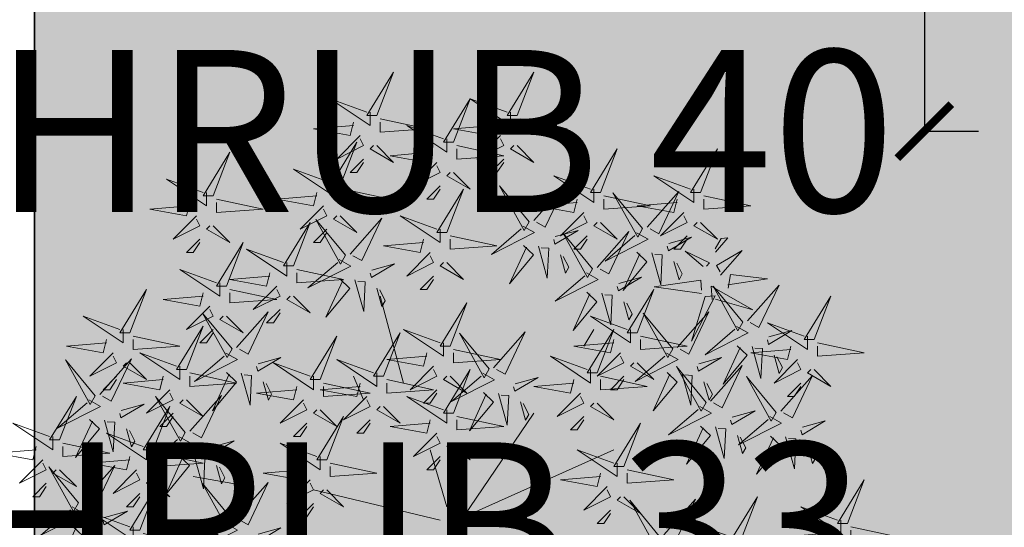
# Model space of a CAD drawing. Units: inches. Extents: x 1704 to 6393, y -157 to 1172.
# Tile 13 of 122: x 1898 to 1934, y 138 to 157. Entities that reach past the tile are written whole.
import ezdxf

# ---------------------------------------------------------------- set-up
doc = ezdxf.new("R2010")
doc.units = ezdxf.units.IN
doc.header["$MEASUREMENT"] = 0
for name, color, linetype, lineweight in [('A-ANNO-DIMS', 7, 'Continuous', 13), ('C-PROP', 7, 'Continuous', 35), ('L-shrub', 74, 'Continuous', 18)]:
    doc.layers.add(name, color=color, linetype=linetype, lineweight=lineweight)
doc.layers.add('L-PLNT-PATT', color=253, linetype='Continuous', lineweight=13, true_color=0x9abc8f)
doc.styles.get("Standard").update_dxf_attribs({"font": 'arial.ttf'})
doc.dimstyles.get("Standard").update_dxf_attribs({"dimtxt": 6, "dimasz": 2, "dimexe": 0.18, "dimexo": 0.0625, "dimgap": 0.09, "dimtad": 0, "dimtih": 1, "dimtoh": 1, "dimdec": 1, "dimzin": 0, "dimdsep": 46, "dimlunit": 3, "dimtxsty": 'Standard', "dimblk": 'ARCHTICK', "dimcen": 0.09, "dimadec": 0, "dimazin": 0, "dimtfac": 1, "dimtdec": 1, "dimtofl": 0, "dimtmove": 0, "dimatfit": 3, "dimfxl": 1, "dimtolj": 1, "dimtzin": 0, "dimarcsym": 0})

# ---------------------------------------------------------------- blocks, each defined once
blk = doc.blocks.new('autumn shrub')
at = {"layer": 'L-shrub'}
for p, q in [((11.54, 1.92), (51.94, 98)), ((1.92, -3.84), (-38.48, 86.47)), ((-98.12, 69.17), (-107.74, 74.94)), ((0, 0), (-59.64, 40.35)), ((71.18, 17.29), (98.12, 26.9)), ((9.62, -3.84), (71.18, 17.29)), ((11.54, -5.76), (55.79, 0)), ((-5.77, -9.61), (-38.48, -19.21)), ((1.92, -13.45), (-15.39, -86.47)), ((17.31, -26.9), (25.01, -40.35)), ((-76.95, -34.59), (-126.97, -48.04)), ((-67.33, -57.64), (-80.8, -63.41)), ((46.17, -69.17), (63.49, -101.84)), ((-17.31, -122.97), (-23.09, -155.64))]:
    blk.add_line(p, q, dxfattribs=at)
for points in [[(5.77, 222.89), (11.54, 249.79), (13.47, 222.89), (7.7, 222.89)], [(-100.04, 203.68), (-94.27, 230.58), (-92.34, 203.68), (-98.12, 203.68)], [(3.85, 220.97), (-21.16, 230.58), (3.85, 215.21), (3.85, 220.97)], [(21.16, 220.97), (30.78, 230.58), (23.09, 217.13), (21.16, 219.05)], [(1.92, 217.13), (9.62, 217.13), (-5.77, 194.07), (1.92, 215.21)], [(98.12, 194.07), (103.89, 220.97), (105.81, 194.07), (100.04, 194.07)], [(-101.96, 201.75), (-126.97, 211.36), (-101.96, 195.99), (-101.96, 201.75)], [(-84.65, 201.75), (-75.03, 211.36), (-82.73, 197.91), (-84.65, 199.83)], [(15.39, 211.36), (28.86, 197.91), (21.16, 213.28), (17.31, 211.36)], [(28.86, 213.28), (36.55, 205.6), (36.55, 209.44), (30.78, 213.28)], [(-51.51, 194.97), (-55.15, 208.07), (-47.22, 194.76), (-49.84, 194.03)], [(7.7, 207.52), (15.39, 205.6), (11.54, 184.46), (9.62, 207.52)], [(46.17, 180.62), (51.94, 207.52), (53.87, 180.62), (48.1, 180.62)], [(-60.75, 182.51), (-81.34, 200.76), (-56.96, 189.22), (-59.8, 184.19)], [(-41.04, 197.9), (-30.56, 200.83), (-33.91, 202.71), (-40.09, 199.58)], [(96.19, 192.15), (71.18, 201.75), (96.19, 186.38), (96.19, 192.15)], [(113.51, 192.15), (123.13, 201.75), (115.43, 188.3), (113.51, 190.23)], [(-103.89, 197.91), (-96.19, 197.91), (-111.58, 174.85), (-103.89, 195.99)], [(-90.42, 192.15), (-76.95, 178.7), (-84.65, 194.07), (-88.5, 192.15)], [(-76.95, 194.07), (-69.26, 186.38), (-69.26, 190.23), (-75.03, 194.07)], [(-103.45, 175.76), (-107.1, 188.86), (-99.16, 175.55), (-101.78, 174.81)], [(-98.12, 188.3), (-90.42, 186.38), (-94.27, 165.25), (-96.19, 188.3)], [(-45.98, 185.23), (-27.65, 190.35), (-44.82, 191.2), (-45.03, 186.9)], [(15.39, 161.4), (21.16, 188.3), (23.09, 161.4), (17.31, 161.4)], [(44.25, 178.7), (19.24, 188.3), (44.25, 172.93), (44.25, 178.7)], [(61.56, 178.7), (71.18, 188.3), (63.49, 174.85), (61.56, 176.78)], [(94.27, 188.3), (101.96, 188.3), (86.57, 165.25), (94.27, 186.38)], [(-112.69, 163.3), (-133.28, 181.54), (-108.91, 170), (-111.74, 164.97)], [(-92.98, 178.69), (-82.5, 181.61), (-85.85, 183.5), (-92.03, 180.36)], [(-57.62, 176.33), (-53.83, 183.03), (-41.31, 158.3), (-55.94, 175.38)], [(-46.41, 176.64), (-40.96, 182.39), (-24.44, 168.66), (-45.47, 178.31)], [(107.74, 182.54), (121.2, 169.09), (113.51, 184.46), (109.66, 182.54)], [(121.2, 184.46), (128.9, 176.78), (128.9, 180.62), (123.13, 184.46)], [(138.52, 155.64), (144.29, 182.54), (146.21, 155.64), (140.44, 155.64)], [(-60.02, 179.89), (-80.67, 162.83), (-55, 177.06), (-60.02, 179.89)], [(100.04, 178.7), (107.74, 176.78), (103.89, 155.64), (101.96, 178.7)], [(-131.51, 152.18), (-139.33, 153.55), (-136.98, 174.91), (-133.43, 152.04)], [(-97.92, 166.01), (-79.59, 171.13), (-96.76, 171.98), (-96.98, 167.69)], [(42.32, 174.85), (50.02, 174.85), (34.63, 151.8), (42.32, 172.93)], [(55.79, 169.09), (69.26, 155.64), (61.56, 171.01), (57.72, 169.09)], [(69.26, 171.01), (76.95, 163.33), (76.95, 167.17), (71.18, 171.01)], [(-184.69, 138.35), (-178.92, 165.25), (-176.99, 138.35), (-182.77, 138.35)], [(-125.08, 143), (-132.76, 142.46), (-119.03, 166.55), (-125.21, 144.92)], [(-57.28, 154.62), (-60.92, 167.72), (-52.99, 154.41), (-55.61, 153.68)], [(13.47, 159.48), (-11.54, 169.09), (13.47, 153.72), (13.47, 159.48)], [(30.78, 159.48), (40.4, 169.09), (32.71, 155.64), (30.78, 157.56)], [(48.1, 165.25), (55.79, 163.33), (51.94, 142.19), (50.02, 165.25)], [(57.72, 140.27), (63.49, 167.17), (65.41, 140.27), (59.64, 140.27)], [(-138.92, 147.8), (-153.3, 160.27), (-144.54, 145.48), (-140.84, 147.67)], [(-111.96, 160.68), (-132.62, 143.61), (-106.94, 157.85), (-111.96, 160.68)], [(-109.56, 157.11), (-105.78, 163.82), (-93.26, 139.08), (-107.89, 156.17)], [(-98.36, 157.42), (-92.9, 163.18), (-76.38, 149.44), (-97.41, 159.1)], [(-66.52, 142.16), (-87.11, 160.4), (-62.74, 148.86), (-65.57, 143.84)], [(-46.81, 157.55), (-36.33, 160.48), (-39.68, 162.36), (-45.86, 159.22)], [(136.59, 153.72), (111.58, 163.33), (136.59, 147.95), (136.59, 153.72)], [(153.91, 153.72), (163.53, 163.33), (155.83, 149.87), (153.91, 151.8)], [(11.54, 155.64), (19.24, 155.64), (3.85, 132.58), (11.54, 153.72)], [(-152.22, 144.94), (-160.44, 152.06), (-160.16, 148.23), (-154.14, 144.8)], [(-88.06, 135.41), (-91.71, 148.51), (-83.77, 135.2), (-86.39, 134.46)], [(-51.75, 144.88), (-33.42, 150), (-50.59, 150.85), (-50.8, 146.55)], [(25.01, 149.87), (38.48, 136.42), (30.78, 151.8), (26.93, 149.87)], [(55.79, 138.35), (30.78, 147.95), (55.79, 132.58), (55.79, 138.35)], [(38.48, 151.8), (46.17, 144.11), (46.17, 147.95), (40.4, 151.8)], [(73.11, 138.35), (82.73, 147.95), (75.03, 134.5), (73.11, 136.42)], [(134.67, 149.87), (142.36, 149.87), (126.97, 126.82), (134.67, 147.95)], [(150.06, 122.97), (155.83, 149.87), (157.76, 122.97), (151.98, 122.97)], [(-186.61, 136.42), (-211.62, 146.03), (-186.61, 130.66), (-186.61, 136.42)], [(-169.3, 136.42), (-159.68, 146.03), (-167.38, 132.58), (-169.3, 134.5)], [(-126.73, 139.03), (-101.1, 131.22), (-127.13, 144.78), (-126.73, 139.03)], [(-77.59, 138.33), (-67.11, 141.26), (-70.46, 143.15), (-76.64, 140.01)], [(-63.39, 135.98), (-59.61, 142.68), (-47.08, 117.95), (-61.71, 135.03)], [(-52.18, 136.28), (-46.73, 142.04), (-30.21, 128.31), (-51.24, 137.96)], [(17.31, 146.03), (25.01, 144.11), (21.16, 122.97), (19.24, 146.03)], [(148.14, 144.11), (161.6, 130.66), (153.91, 146.03), (150.06, 144.11)], [(161.6, 146.03), (169.3, 138.35), (169.3, 142.19), (163.53, 146.03)], [(-144, 137.81), (-152.92, 127.55), (-146.19, 141.51), (-144.13, 139.73)], [(-128.51, 136.98), (-132.37, 109.74), (-136.19, 136.44), (-130.43, 136.85)], [(-97.3, 122.95), (-117.89, 141.19), (-93.52, 129.65), (-96.35, 124.62)], [(-65.79, 139.54), (-86.44, 122.48), (-60.77, 136.71), (-65.79, 139.54)], [(19.67, 127.72), (16.03, 140.82), (23.96, 127.51), (21.35, 126.78)], [(108.17, 127.72), (104.53, 140.82), (112.46, 127.51), (109.84, 126.78)], [(140.44, 140.27), (148.14, 138.35), (144.29, 117.21), (142.36, 140.27)], [(-188.54, 132.58), (-180.84, 132.58), (-196.23, 109.52), (-188.54, 130.66)], [(-157.32, 118.11), (-160.96, 131.21), (-153.03, 117.9), (-155.65, 117.17)], [(-82.53, 125.66), (-64.2, 130.78), (-81.37, 131.63), (-81.59, 127.34)], [(10.44, 115.26), (-10.16, 133.5), (14.22, 121.96), (11.38, 116.94)], [(30.15, 130.65), (40.62, 133.58), (37.28, 135.46), (31.09, 132.32)], [(53.87, 134.5), (61.56, 134.5), (46.17, 111.45), (53.87, 132.58)], [(67.33, 128.74), (80.8, 115.29), (73.11, 130.66), (69.26, 128.74)], [(98.93, 115.26), (78.34, 133.5), (102.71, 121.96), (99.88, 116.94)], [(78.88, 103.76), (84.65, 130.66), (86.57, 103.76), (80.8, 103.76)], [(80.8, 130.66), (88.5, 122.97), (88.5, 126.82), (82.73, 130.66)], [(118.64, 130.65), (129.12, 133.58), (125.77, 135.46), (119.59, 132.32)], [(148.14, 121.05), (123.13, 130.66), (148.14, 115.29), (148.14, 121.05)], [(165.45, 121.05), (175.07, 130.66), (167.38, 117.21), (165.45, 119.13)], [(-175.07, 126.82), (-161.6, 113.37), (-169.3, 128.74), (-173.15, 126.82)], [(-161.6, 128.74), (-153.91, 121.05), (-153.91, 124.9), (-159.68, 128.74)], [(-146.85, 121.04), (-136.37, 123.97), (-139.72, 125.86), (-145.9, 122.72)], [(-103.89, 101.84), (-98.12, 128.74), (-96.19, 101.84), (-101.96, 101.84)], [(59.64, 124.9), (67.33, 122.97), (63.49, 101.84), (61.56, 124.9)], [(-166.56, 105.65), (-187.15, 123.9), (-162.78, 112.36), (-165.61, 107.33)], [(-182.77, 122.97), (-175.07, 121.05), (-178.92, 99.92), (-180.84, 122.97)], [(-96.57, 120.33), (-117.23, 103.26), (-91.55, 117.49), (-96.57, 120.33)], [(-94.17, 116.76), (-90.39, 123.47), (-77.87, 98.73), (-92.49, 115.82)], [(-82.96, 117.07), (-77.51, 122.83), (-60.99, 109.09), (-82.02, 118.75)], [(-26.93, 94.15), (-21.16, 121.05), (-19.24, 94.15), (-25.01, 94.15)], [(25.2, 117.98), (43.54, 123.1), (26.37, 123.95), (26.15, 119.65)], [(113.7, 117.98), (132.03, 123.1), (114.86, 123.95), (114.65, 119.65)], [(200.08, 94.15), (205.85, 121.05), (207.78, 94.15), (202, 94.15)], [(-151.79, 108.37), (-133.46, 113.49), (-150.63, 114.34), (-150.84, 110.04)], [(13.57, 109.08), (17.35, 115.78), (29.87, 91.05), (15.24, 108.13)], [(24.77, 109.38), (30.23, 115.14), (46.74, 101.41), (25.72, 111.06)], [(102.06, 109.08), (105.85, 115.78), (118.37, 91.05), (103.74, 108.13)], [(113.27, 109.38), (118.72, 115.14), (135.24, 101.41), (114.21, 111.06)], [(146.21, 117.21), (153.91, 117.21), (138.52, 94.15), (146.21, 115.29)], [(159.68, 111.45), (173.15, 98), (165.45, 113.37), (161.6, 111.45)], [(173.15, 113.37), (180.84, 105.68), (180.84, 109.52), (175.07, 113.37)], [(-105.81, 99.92), (-130.82, 109.52), (-105.81, 94.15), (-105.81, 99.92)], [(-88.5, 99.92), (-78.88, 109.52), (-86.57, 96.07), (-88.5, 98)], [(11.17, 112.64), (-9.49, 95.58), (16.19, 109.81), (11.17, 112.64)], [(76.95, 101.84), (51.94, 111.45), (76.95, 96.07), (76.95, 101.84)], [(99.66, 112.64), (79.01, 95.58), (104.68, 109.81), (99.66, 112.64)], [(94.27, 101.84), (103.89, 111.45), (96.19, 98), (94.27, 99.92)], [(-165.83, 103.03), (-186.48, 85.97), (-160.81, 100.2), (-165.83, 103.03)], [(-184.69, 80.7), (-178.92, 107.6), (-176.99, 80.7), (-182.77, 80.7)], [(-163.43, 99.47), (-159.65, 106.17), (-147.12, 81.44), (-161.75, 98.53)], [(-152.22, 99.78), (-146.77, 105.54), (-130.25, 91.8), (-151.28, 101.45)], [(-134.24, 89.29), (-137.88, 102.39), (-129.94, 89.08), (-132.56, 88.35)], [(-80.8, 78.78), (-75.03, 105.68), (-73.11, 78.78), (-78.88, 78.78)], [(134.67, 76.86), (140.44, 103.76), (142.36, 76.86), (136.59, 76.86)], [(151.98, 107.6), (159.68, 105.68), (155.83, 84.54), (153.91, 107.6)], [(-123.76, 92.22), (-113.29, 95.15), (-116.63, 97.03), (-122.82, 93.89)], [(-28.86, 92.23), (-53.87, 101.84), (-28.86, 86.47), (-28.86, 92.23)], [(-11.54, 92.23), (-1.92, 101.84), (-9.62, 88.39), (-11.54, 90.31)], [(75.03, 98), (82.73, 98), (67.33, 74.94), (75.03, 96.07)], [(75.03, 71.09), (80.8, 98), (82.73, 71.09), (76.95, 71.09)], [(198.16, 92.23), (173.15, 101.84), (198.16, 86.47), (198.16, 92.23)], [(215.47, 92.23), (225.09, 101.84), (217.4, 88.39), (215.47, 90.31)], [(-143.47, 76.83), (-164.07, 95.07), (-139.69, 83.53), (-142.53, 78.51)], [(-107.74, 96.07), (-100.04, 96.07), (-115.43, 73.02), (-107.74, 94.15)], [(-94.27, 90.31), (-80.8, 76.86), (-88.5, 92.23), (-92.34, 90.31)], [(-80.8, 92.23), (-73.11, 84.54), (-73.11, 88.39), (-78.88, 92.23)], [(88.5, 92.23), (101.96, 78.78), (94.27, 94.15), (90.42, 92.23)], [(101.96, 94.15), (109.66, 86.47), (109.66, 90.31), (103.89, 94.15)], [(-186.61, 78.78), (-211.62, 88.39), (-186.61, 73.02), (-186.61, 78.78)], [(-169.3, 78.78), (-159.68, 88.39), (-167.38, 74.94), (-169.3, 76.86)], [(-128.7, 79.55), (-110.37, 84.67), (-127.54, 85.52), (-127.76, 81.22)], [(-82.73, 76.86), (-107.74, 86.47), (-82.73, 71.09), (-82.73, 76.86)], [(-101.96, 86.47), (-94.27, 84.54), (-98.12, 63.41), (-100.04, 86.47)], [(-65.41, 76.86), (-55.79, 86.47), (-63.49, 73.02), (-65.41, 74.94)], [(-30.78, 88.39), (-23.09, 88.39), (-38.48, 65.33), (-30.78, 86.47)], [(80.8, 88.39), (88.5, 86.47), (84.65, 65.33), (82.73, 88.39)], [(196.23, 88.39), (203.93, 88.39), (188.54, 65.33), (196.23, 86.47)], [(-17.31, 82.62), (-3.85, 69.17), (-11.54, 84.54), (-15.39, 82.62)], [(-3.85, 84.54), (3.85, 76.86), (3.85, 80.7), (-1.92, 84.54)], [(44.25, 57.64), (50.02, 84.54), (51.94, 57.64), (46.17, 57.64)], [(98.12, 53.8), (103.89, 80.7), (105.81, 53.8), (100.04, 53.8)], [(132.75, 74.94), (107.74, 84.54), (132.75, 69.17), (132.75, 74.94)], [(150.06, 74.94), (159.68, 84.54), (151.98, 71.09), (150.06, 73.02)], [(190.46, 53.8), (196.23, 80.7), (198.16, 53.8), (192.39, 53.8)], [(209.7, 82.62), (223.17, 69.17), (215.47, 84.54), (211.62, 82.62)], [(223.17, 84.54), (230.86, 76.86), (230.86, 80.7), (225.09, 84.54)], [(-188.54, 74.94), (-180.84, 74.94), (-196.23, 51.88), (-188.54, 73.02)], [(-142.74, 74.21), (-163.4, 57.15), (-137.72, 71.38), (-142.74, 74.21)], [(-140.34, 70.65), (-136.56, 77.35), (-124.04, 52.62), (-138.67, 69.7)], [(-129.14, 70.95), (-123.68, 76.71), (-107.16, 62.98), (-128.19, 72.63)], [(-25.01, 78.78), (-17.31, 76.86), (-21.16, 55.72), (-23.09, 78.78)], [(42.76, 62.39), (39.12, 75.49), (47.05, 62.18), (44.43, 61.45)], [(73.11, 69.17), (48.1, 78.78), (73.11, 63.41), (73.11, 69.17)], [(90.42, 69.17), (100.04, 78.78), (92.34, 65.33), (90.42, 67.25)], [(202, 78.78), (209.7, 76.86), (205.85, 55.72), (203.93, 78.78)], [(-175.07, 69.17), (-161.6, 55.72), (-169.3, 71.09), (-173.15, 69.17)], [(-161.6, 71.09), (-153.91, 63.41), (-153.91, 67.25), (-159.68, 71.09)], [(-84.65, 73.02), (-76.95, 73.02), (-92.34, 49.96), (-84.65, 71.09)], [(-71.18, 67.25), (-57.72, 53.8), (-65.41, 69.17), (-69.26, 67.25)], [(-57.72, 69.17), (-50.02, 61.49), (-50.02, 65.33), (-55.79, 69.17)], [(33.52, 49.93), (12.93, 68.17), (37.3, 56.63), (34.47, 51.61)], [(53.23, 65.32), (63.71, 68.25), (60.36, 70.13), (54.18, 66.99)], [(130.82, 71.09), (138.52, 71.09), (123.13, 48.04), (130.82, 69.17)], [(-182.77, 65.33), (-175.07, 63.41), (-178.92, 42.27), (-180.84, 65.33)], [(-161.17, 52.78), (-164.81, 65.88), (-156.88, 52.57), (-159.5, 51.84)], [(-78.88, 63.41), (-71.18, 61.49), (-75.03, 40.35), (-76.95, 63.41)], [(42.32, 55.72), (17.31, 65.33), (42.32, 49.96), (42.32, 55.72)], [(59.64, 55.72), (69.26, 65.33), (61.56, 51.88), (59.64, 53.8)], [(71.18, 65.33), (78.88, 65.33), (63.49, 42.27), (71.18, 63.41)], [(144.29, 65.33), (157.76, 51.88), (150.06, 67.25), (146.21, 65.33)], [(157.76, 67.25), (165.45, 59.57), (165.45, 63.41), (159.68, 67.25)], [(-228.94, 32.67), (-223.17, 59.57), (-221.24, 32.67), (-227.01, 32.67)], [(-170.4, 40.32), (-191, 58.57), (-166.62, 47.03), (-169.46, 42)], [(-150.69, 55.71), (-140.22, 58.64), (-143.57, 60.53), (-149.75, 57.39)], [(48.29, 52.64), (66.62, 57.77), (49.45, 58.62), (49.24, 54.32)], [(96.19, 51.88), (71.18, 61.49), (96.19, 46.12), (96.19, 51.88)], [(84.65, 59.57), (98.12, 46.12), (90.42, 61.49), (86.57, 59.57)], [(98.12, 61.49), (105.81, 53.8), (105.81, 57.64), (100.04, 61.49)], [(113.51, 51.88), (123.13, 61.49), (115.43, 48.04), (113.51, 49.96)], [(136.59, 61.49), (144.29, 59.57), (140.44, 38.43), (138.52, 61.49)], [(188.54, 51.88), (163.53, 61.49), (188.54, 46.12), (188.54, 51.88)], [(184.69, 30.74), (190.46, 57.64), (192.39, 30.74), (186.61, 30.74)], [(205.85, 51.88), (215.47, 61.49), (207.78, 48.04), (205.85, 49.96)], [(227.01, 32.67), (232.79, 59.57), (234.71, 32.67), (228.94, 32.67)], [(40.4, 51.88), (48.1, 51.88), (32.71, 28.82), (40.4, 49.96)], [(76.95, 55.72), (84.65, 53.8), (80.8, 32.67), (78.88, 55.72)], [(-155.64, 43.04), (-137.31, 48.16), (-154.48, 49.01), (-154.69, 44.71)], [(34.25, 47.31), (13.6, 30.25), (39.27, 44.48), (34.25, 47.31)], [(36.65, 43.75), (40.43, 50.45), (52.96, 25.72), (38.33, 42.8)], [(47.86, 44.05), (53.31, 49.81), (69.83, 36.08), (48.8, 45.73)], [(53.87, 46.12), (67.33, 32.67), (59.64, 48.04), (55.79, 46.12)], [(67.33, 48.04), (75.03, 40.35), (75.03, 44.19), (69.26, 48.04)], [(94.27, 48.04), (101.96, 48.04), (86.57, 24.98), (94.27, 46.12)], [(186.61, 48.04), (194.31, 48.04), (178.92, 24.98), (186.61, 46.12)], [(-230.86, 30.74), (-255.87, 40.35), (-230.86, 24.98), (-230.86, 30.74)], [(-213.55, 30.74), (-203.93, 40.35), (-211.62, 26.9), (-213.55, 28.82)], [(-167.27, 34.14), (-163.49, 40.84), (-150.97, 16.11), (-165.6, 33.2)], [(-156.07, 34.45), (-150.62, 40.21), (-134.1, 26.47), (-155.13, 36.12)], [(-76.52, 29.73), (-80.16, 42.83), (-72.23, 29.51), (-74.85, 28.78)], [(46.17, 42.27), (53.87, 40.35), (50.02, 19.21), (48.1, 42.27)], [(107.74, 42.27), (121.2, 28.82), (113.51, 44.19), (109.66, 42.27)], [(121.2, 44.19), (128.9, 36.51), (128.9, 40.35), (123.13, 44.19)], [(154.34, 31.65), (150.7, 44.75), (158.63, 31.44), (156.02, 30.7)], [(200.08, 42.27), (213.55, 28.82), (205.85, 44.19), (202, 42.27)], [(225.09, 30.74), (200.08, 40.35), (225.09, 24.98), (225.09, 30.74)], [(213.55, 44.19), (221.24, 36.51), (221.24, 40.35), (215.47, 44.19)], [(242.41, 30.74), (252.02, 40.35), (244.33, 26.9), (242.41, 28.82)], [(-169.68, 37.7), (-190.33, 20.64), (-164.66, 34.87), (-169.68, 37.7)], [(-85.76, 17.27), (-106.35, 35.51), (-81.97, 23.97), (-84.81, 18.94)], [(-66.05, 32.65), (-55.57, 35.58), (-58.92, 37.47), (-65.1, 34.33)], [(100.04, 38.43), (107.74, 36.51), (103.89, 15.37), (101.96, 38.43)], [(145.11, 19.19), (124.51, 37.43), (148.89, 25.89), (146.05, 20.86)], [(182.77, 28.82), (157.76, 38.43), (182.77, 23.06), (182.77, 28.82)], [(164.82, 34.57), (175.29, 37.5), (171.94, 39.39), (165.76, 36.25)], [(192.39, 38.43), (200.08, 36.51), (196.23, 15.37), (194.31, 38.43)], [(200.08, 28.82), (209.7, 38.43), (202, 24.98), (200.08, 26.9)], [(-232.79, 26.9), (-225.09, 26.9), (-240.48, 3.84), (-232.79, 24.98)], [(-219.32, 21.14), (-205.85, 7.69), (-213.55, 23.06), (-217.4, 21.14)], [(-213.55, -3.84), (-207.78, 23.06), (-205.85, -3.84), (-211.62, -3.84)], [(-205.85, 23.06), (-198.16, 15.37), (-198.16, 19.21), (-203.93, 23.06)], [(-70.99, 19.98), (-52.66, 25.1), (-69.83, 25.95), (-70.04, 21.66)], [(-57.72, -3.84), (-51.94, 23.06), (-50.02, -3.84), (-55.79, -3.84)], [(159.87, 21.9), (178.21, 27.02), (161.04, 27.87), (160.82, 23.58)], [(180.84, 24.98), (188.54, 24.98), (173.15, 1.92), (180.84, 23.06)], [(223.17, 26.9), (230.86, 26.9), (215.47, 3.84), (223.17, 24.98)], [(215.47, -1.92), (221.24, 24.98), (223.17, -1.92), (217.4, -1.92)], [(236.63, 21.14), (250.1, 7.69), (242.41, 23.06), (238.56, 21.14)], [(250.1, 23.06), (257.8, 15.37), (257.8, 19.21), (252.02, 23.06)], [(-227.01, 17.29), (-219.32, 15.37), (-223.17, -5.76), (-225.09, 17.29)], [(-161.6, -7.69), (-155.83, 19.21), (-153.91, -7.69), (-159.68, -7.69)], [(-96.19, -5.76), (-90.42, 21.14), (-88.5, -5.76), (-94.27, -5.76)], [(-82.63, 11.08), (-78.84, 17.78), (-66.32, -6.95), (-80.95, 10.14)], [(-71.42, 11.39), (-65.97, 17.15), (-49.45, 3.41), (-70.48, 13.06)], [(34.63, -9.61), (40.4, 17.29), (42.32, -9.61), (36.55, -9.61)], [(148.24, 13), (152.02, 19.71), (164.54, -5.03), (149.91, 12.06)], [(159.44, 13.31), (164.89, 19.07), (181.41, 5.33), (160.39, 14.99)], [(194.31, 19.21), (207.78, 5.76), (200.08, 21.14), (196.23, 19.21)], [(207.78, 21.14), (215.47, 13.45), (215.47, 17.29), (209.7, 21.14)], [(228.94, 17.29), (236.63, 15.37), (232.79, -5.76), (230.86, 17.29)], [(-85.03, 14.65), (-105.68, -2.42), (-80.01, 11.81), (-85.03, 14.65)], [(145.83, 16.57), (125.18, -0.5), (150.86, 13.74), (145.83, 16.57)], [(186.61, 15.37), (194.31, 13.45), (190.46, -7.69), (188.54, 15.37)], [(213.55, -3.84), (188.54, 5.76), (213.55, -9.61), (213.55, -3.84)], [(230.86, -3.84), (240.48, 5.76), (232.79, -7.69), (230.86, -5.76)], [(-215.47, -5.76), (-240.48, 3.84), (-215.47, -11.53), (-215.47, -5.76)], [(-198.16, -5.76), (-188.54, 3.84), (-196.23, -9.61), (-198.16, -7.69)], [(-163.53, -9.61), (-188.54, 0), (-163.53, -15.37), (-163.53, -9.61)], [(-146.21, -9.61), (-136.59, 0), (-144.29, -13.45), (-146.21, -11.53)], [(-98.12, -7.69), (-123.13, 1.92), (-98.12, -13.45), (-98.12, -7.69)], [(-59.64, -5.76), (-84.65, 3.84), (-59.64, -11.53), (-59.64, -5.76)], [(-80.8, -7.69), (-71.18, 1.92), (-78.88, -11.53), (-80.8, -9.61)], [(-42.32, -5.76), (-32.71, 3.84), (-40.4, -9.61), (-42.32, -7.69)], [(110.09, -10.62), (106.45, 2.47), (114.39, -10.84), (111.77, -11.57)], [(232.79, -26.9), (238.56, 0), (240.48, -26.9), (234.71, -26.9)], [(32.71, -11.53), (7.7, -1.92), (32.71, -17.29), (32.71, -11.53)], [(50.02, -11.53), (59.64, -1.92), (51.94, -15.37), (50.02, -13.45)], [(100.86, -23.09), (80.26, -4.84), (104.64, -16.38), (101.8, -21.41)], [(120.57, -7.7), (131.04, -4.77), (127.7, -2.88), (121.51, -6.02)], [(-217.4, -9.61), (-209.7, -9.61), (-225.09, -32.67), (-217.4, -11.53)], [(-61.56, -9.61), (-53.87, -9.61), (-69.26, -32.67), (-61.56, -11.53)], [(211.62, -7.69), (219.32, -7.69), (203.93, -30.74), (211.62, -9.61)], [(-203.93, -15.37), (-190.46, -28.82), (-198.16, -13.45), (-202, -15.37)], [(-190.46, -13.45), (-182.77, -21.14), (-182.77, -17.29), (-188.54, -13.45)], [(-165.45, -13.45), (-157.76, -13.45), (-173.15, -36.51), (-165.45, -15.37)], [(-100.04, -11.53), (-92.34, -11.53), (-107.74, -34.59), (-100.04, -13.45)], [(-86.57, -17.29), (-73.11, -30.74), (-80.8, -15.37), (-84.65, -17.29)], [(-73.11, -15.37), (-65.41, -23.06), (-65.41, -19.21), (-71.18, -15.37)], [(-48.1, -15.37), (-34.63, -28.82), (-42.32, -13.45), (-46.17, -15.37)], [(-34.63, -13.45), (-26.93, -21.14), (-26.93, -17.29), (-32.71, -13.45)], [(30.78, -15.37), (38.48, -15.37), (23.09, -38.43), (30.78, -17.29)], [(115.63, -20.37), (133.96, -15.25), (116.79, -14.4), (116.57, -18.7)], [(225.09, -13.45), (238.56, -26.9), (230.86, -11.53), (227.01, -13.45)], [(238.56, -11.53), (246.25, -19.21), (246.25, -15.37), (240.48, -11.53)], [(-228.94, -48.04), (-223.17, -21.14), (-221.24, -48.04), (-227.01, -48.04)], [(-211.62, -19.21), (-203.93, -21.14), (-207.78, -42.27), (-209.7, -19.21)], [(-151.98, -19.21), (-138.52, -32.67), (-146.21, -17.29), (-150.06, -19.21)], [(-138.52, -17.29), (-130.82, -24.98), (-130.82, -21.14), (-136.59, -17.29)], [(-94.27, -21.14), (-86.57, -23.06), (-90.42, -44.19), (-92.34, -21.14)], [(-78.88, -44.19), (-73.11, -17.29), (-71.18, -44.19), (-76.95, -44.19)], [(-55.79, -19.21), (-48.1, -21.14), (-51.94, -42.27), (-53.87, -19.21)], [(44.25, -21.14), (57.72, -34.59), (50.02, -19.21), (46.17, -21.14)], [(57.72, -19.21), (65.41, -26.9), (65.41, -23.06), (59.64, -19.21)], [(103.99, -29.27), (107.77, -22.57), (120.29, -47.3), (105.66, -30.21)], [(230.86, -28.82), (205.85, -19.21), (230.86, -34.59), (230.86, -28.82)], [(217.4, -17.29), (225.09, -19.21), (221.24, -40.35), (219.32, -17.29)], [(248.18, -28.82), (257.8, -19.21), (250.1, -32.67), (248.18, -30.74)], [(-159.68, -23.06), (-151.98, -24.98), (-155.83, -46.12), (-157.76, -23.06)], [(36.55, -24.98), (44.25, -26.9), (40.4, -48.04), (38.48, -24.98)], [(71.18, -53.8), (76.95, -26.9), (78.88, -53.8), (73.11, -53.8)], [(101.59, -25.71), (80.93, -42.77), (106.61, -28.54), (101.59, -25.71)], [(115.19, -28.96), (120.65, -23.2), (137.17, -36.94), (116.14, -27.29)], [(40.4, -59.57), (46.17, -32.67), (48.1, -59.57), (42.32, -59.57)], [(173.15, -55.72), (178.92, -28.82), (180.84, -55.72), (175.07, -55.72)], [(228.94, -32.67), (236.63, -32.67), (221.24, -55.72), (228.94, -34.59)], [(-80.8, -46.12), (-105.81, -36.51), (-80.8, -51.88), (-80.8, -46.12)], [(-63.49, -46.12), (-53.87, -36.51), (-61.56, -49.96), (-63.49, -48.04)], [(111.58, -61.49), (117.35, -34.59), (119.28, -61.49), (113.51, -61.49)], [(242.41, -38.43), (255.87, -51.88), (248.18, -36.51), (244.33, -38.43)], [(255.87, -36.51), (263.57, -44.19), (263.57, -40.35), (257.8, -36.51)], [(-230.86, -49.96), (-255.87, -40.35), (-230.86, -55.72), (-230.86, -49.96)], [(-213.55, -49.96), (-203.93, -40.35), (-211.62, -53.8), (-213.55, -51.88)], [(-188.54, -69.17), (-182.77, -42.27), (-180.84, -69.17), (-186.61, -69.17)], [(-141.93, -52.9), (-145.57, -39.8), (-137.64, -53.11), (-140.26, -53.84)], [(-131.46, -49.97), (-120.98, -47.04), (-124.33, -45.16), (-130.51, -48.29)], [(234.71, -42.27), (242.41, -44.19), (238.56, -65.33), (236.63, -42.27)], [(-151.17, -65.36), (-171.76, -47.11), (-147.39, -58.66), (-150.22, -63.68)], [(-82.73, -49.96), (-75.03, -49.96), (-90.42, -73.02), (-82.73, -51.88)], [(-30.78, -76.86), (-25.01, -49.96), (-23.09, -76.86), (-28.86, -76.86)], [(69.26, -55.72), (44.25, -46.12), (69.26, -61.49), (69.26, -55.72)], [(86.57, -55.72), (96.19, -46.12), (88.5, -59.57), (86.57, -57.64)], [(171.22, -57.64), (146.21, -48.04), (171.22, -63.41), (171.22, -57.64)], [(188.54, -57.64), (198.16, -48.04), (190.46, -61.49), (188.54, -59.57)], [(-232.79, -53.8), (-225.09, -53.8), (-240.48, -76.86), (-232.79, -55.72)], [(-76.95, -80.7), (-71.18, -53.8), (-69.26, -80.7), (-75.03, -80.7)], [(-69.26, -55.72), (-55.79, -69.17), (-63.49, -53.8), (-67.33, -55.72)], [(-55.79, -53.8), (-48.1, -61.49), (-48.1, -57.64), (-53.87, -53.8)], [(38.48, -61.49), (13.47, -51.88), (38.48, -67.25), (38.48, -61.49)], [(55.79, -61.49), (65.41, -51.88), (57.72, -65.33), (55.79, -63.41)], [(109.66, -63.41), (84.65, -53.8), (109.66, -69.17), (109.66, -63.41)], [(126.97, -63.41), (136.59, -53.8), (128.9, -67.25), (126.97, -65.33)], [(211.62, -82.62), (217.4, -55.72), (219.32, -82.62), (213.55, -82.62)], [(-219.32, -59.57), (-205.85, -73.02), (-213.55, -57.64), (-217.4, -59.57)], [(-190.46, -71.09), (-215.47, -61.49), (-190.46, -76.86), (-190.46, -71.09)], [(-205.85, -57.64), (-198.16, -65.33), (-198.16, -61.49), (-203.93, -57.64)], [(-173.15, -71.09), (-163.53, -61.49), (-171.22, -74.94), (-173.15, -73.02)], [(-136.4, -62.64), (-118.07, -57.52), (-135.24, -56.67), (-135.45, -60.97)], [(-76.95, -59.57), (-69.26, -61.49), (-73.11, -82.62), (-75.03, -59.57)], [(67.33, -59.57), (75.03, -59.57), (59.64, -82.62), (67.33, -61.49)], [(71.18, -84.54), (76.95, -57.64), (78.88, -84.54), (73.11, -84.54)], [(169.3, -61.49), (176.99, -61.49), (161.6, -84.54), (169.3, -63.41)], [(-227.01, -63.41), (-219.32, -65.33), (-223.17, -86.47), (-225.09, -63.41)], [(-150.44, -67.98), (-171.09, -85.04), (-145.42, -70.81), (-150.44, -67.98)], [(-148.04, -71.54), (-144.26, -64.84), (-131.73, -89.57), (-146.36, -72.49)], [(-136.83, -71.23), (-131.38, -65.48), (-114.86, -79.21), (-135.89, -69.56)], [(36.55, -65.33), (44.25, -65.33), (28.86, -88.39), (36.55, -67.25)], [(80.8, -65.33), (94.27, -78.78), (86.57, -63.41), (82.73, -65.33)], [(94.27, -63.41), (101.96, -71.09), (101.96, -67.25), (96.19, -63.41)], [(107.74, -67.25), (115.43, -67.25), (100.04, -90.31), (107.74, -69.17)], [(150.49, -79.8), (146.85, -66.7), (154.79, -80.01), (152.17, -80.74)], [(182.77, -67.25), (196.23, -80.7), (188.54, -65.33), (184.69, -67.25)], [(196.23, -65.33), (203.93, -73.02), (203.93, -69.17), (198.16, -65.33)], [(-142.36, -96.07), (-136.59, -69.17), (-134.67, -96.07), (-140.44, -96.07)], [(-78.88, -82.62), (-103.89, -73.02), (-78.88, -88.39), (-78.88, -82.62)], [(-61.56, -82.62), (-51.94, -73.02), (-59.64, -86.47), (-61.56, -84.54)], [(-32.71, -78.78), (-57.72, -69.17), (-32.71, -84.54), (-32.71, -78.78)], [(-15.39, -78.78), (-5.77, -69.17), (-13.47, -82.62), (-15.39, -80.7)], [(50.02, -71.09), (63.49, -84.54), (55.79, -69.17), (51.94, -71.09)], [(63.49, -69.17), (71.18, -76.86), (71.18, -73.02), (65.41, -69.17)], [(73.11, -69.17), (80.8, -71.09), (76.95, -92.23), (75.03, -69.17)], [(121.2, -73.02), (134.67, -86.47), (126.97, -71.09), (123.13, -73.02)], [(134.67, -71.09), (142.36, -78.78), (142.36, -74.94), (136.59, -71.09)], [(160.97, -76.87), (171.44, -73.94), (168.1, -72.06), (161.91, -75.19)], [(175.07, -71.09), (182.77, -73.02), (178.92, -94.15), (176.99, -71.09)], [(-192.39, -74.94), (-184.69, -74.94), (-200.08, -98), (-192.39, -76.86)], [(-178.92, -80.7), (-165.45, -94.15), (-173.15, -78.78), (-176.99, -80.7)], [(-165.45, -78.78), (-157.76, -86.47), (-157.76, -82.62), (-163.53, -78.78)], [(42.32, -74.94), (50.02, -76.86), (46.17, -98), (44.25, -74.94)], [(69.26, -86.47), (44.25, -76.86), (69.26, -92.23), (69.26, -86.47)], [(86.57, -86.47), (96.19, -76.86), (88.5, -90.31), (86.57, -88.39)], [(113.51, -76.86), (121.2, -78.78), (117.35, -99.92), (115.43, -76.86)], [(141.26, -92.26), (120.66, -74.02), (145.04, -85.56), (142.2, -90.58)], [(209.7, -84.54), (184.69, -74.94), (209.7, -90.31), (209.7, -84.54)], [(227.01, -84.54), (236.63, -74.94), (228.94, -88.39), (227.01, -86.47)], [(-186.61, -84.54), (-178.92, -86.47), (-182.77, -107.6), (-184.69, -84.54)], [(-34.63, -82.62), (-26.93, -82.62), (-42.32, -105.68), (-34.63, -84.54)], [(156.03, -89.54), (174.36, -84.42), (157.19, -83.57), (156.97, -87.87)], [(-144.29, -98), (-169.3, -88.39), (-144.29, -103.76), (-144.29, -98)], [(-126.97, -98), (-117.35, -88.39), (-125.05, -101.84), (-126.97, -99.92)], [(-80.8, -86.47), (-73.11, -86.47), (-88.5, -109.52), (-80.8, -88.39)], [(-67.33, -92.23), (-53.87, -105.68), (-61.56, -90.31), (-65.41, -92.23)], [(-53.87, -90.31), (-46.17, -98), (-46.17, -94.15), (-51.94, -90.31)], [(-21.16, -88.39), (-7.7, -101.84), (-15.39, -86.47), (-19.24, -88.39)], [(-7.7, -86.47), (0, -94.15), (0, -90.31), (-5.77, -86.47)], [(67.33, -90.31), (75.03, -90.31), (59.64, -113.37), (67.33, -92.23)], [(186.61, -115.29), (192.39, -88.39), (194.31, -115.29), (188.54, -115.29)], [(207.78, -88.39), (215.47, -88.39), (200.08, -111.45), (207.78, -90.31)], [(-75.03, -96.07), (-67.33, -98), (-71.18, -119.13), (-73.11, -96.07)], [(-28.86, -92.23), (-21.16, -94.15), (-25.01, -115.29), (-26.93, -92.23)], [(80.8, -96.07), (94.27, -109.52), (86.57, -94.15), (82.73, -96.07)], [(94.27, -94.15), (101.96, -101.84), (101.96, -98), (96.19, -94.15)], [(141.99, -94.88), (121.33, -111.94), (147.01, -97.71), (141.99, -94.88)], [(144.39, -98.44), (148.17, -91.74), (160.69, -116.47), (146.06, -99.39)], [(155.59, -98.13), (161.05, -92.38), (177.57, -106.11), (156.54, -96.46)], [(221.24, -94.15), (234.71, -107.6), (227.01, -92.23), (223.17, -94.15)], [(234.71, -92.23), (242.41, -99.92), (242.41, -96.07), (236.63, -92.23)], [(-146.21, -101.84), (-138.52, -101.84), (-153.91, -124.9), (-146.21, -103.76)], [(73.11, -99.92), (80.8, -101.84), (76.95, -122.97), (75.03, -99.92)], [(78.88, -128.74), (84.65, -101.84), (86.57, -128.74), (80.8, -128.74)], [(213.55, -98), (221.24, -99.92), (217.4, -121.05), (215.47, -98)], [(-132.75, -107.6), (-119.28, -121.05), (-126.97, -105.68), (-130.82, -107.6)], [(-130.82, -134.5), (-125.05, -107.6), (-123.13, -134.5), (-128.9, -134.5)], [(-119.28, -105.68), (-111.58, -113.37), (-111.58, -109.52), (-117.35, -105.68)], [(-88.06, -118.23), (-91.71, -105.13), (-83.77, -118.44), (-86.39, -119.17)], [(10.05, -118.23), (6.41, -105.13), (14.35, -118.44), (11.73, -119.17)], [(184.69, -117.21), (159.68, -107.6), (184.69, -122.97), (184.69, -117.21)], [(202, -117.21), (211.62, -107.6), (203.93, -121.05), (202, -119.13)], [(-140.44, -111.45), (-132.75, -113.37), (-136.59, -134.5), (-138.52, -111.45)], [(-97.3, -130.69), (-117.89, -112.44), (-93.52, -123.99), (-96.35, -129.01)], [(-77.59, -115.3), (-67.11, -112.37), (-70.46, -110.49), (-76.64, -113.62)], [(0.82, -130.69), (-19.78, -112.44), (4.6, -123.99), (1.76, -129.01)], [(20.53, -115.3), (31, -112.37), (27.66, -110.49), (21.47, -113.62)], [(127.41, -125.91), (123.77, -112.81), (131.7, -126.12), (129.08, -126.86)], [(-182.77, -142.19), (-176.99, -115.29), (-175.07, -142.19), (-180.84, -142.19)], [(137.88, -122.99), (148.36, -120.06), (145.01, -118.17), (138.83, -121.31)], [(-82.53, -127.97), (-64.2, -122.85), (-81.37, -122), (-81.59, -126.3)], [(15.59, -127.97), (33.92, -122.85), (16.75, -122), (16.53, -126.3)], [(76.95, -130.66), (51.94, -121.05), (76.95, -136.42), (76.95, -130.66)], [(53.87, -146.03), (59.64, -119.13), (61.56, -146.03), (55.79, -146.03)], [(94.27, -130.66), (103.89, -121.05), (96.19, -134.5), (94.27, -132.58)], [(118.17, -138.37), (97.58, -120.13), (121.95, -131.67), (119.12, -136.7)], [(163.53, -146.03), (169.3, -119.13), (171.22, -146.03), (165.45, -146.03)], [(182.77, -121.05), (190.46, -121.05), (175.07, -144.11), (182.77, -122.97)], [(-132.75, -136.42), (-157.76, -126.82), (-132.75, -142.19), (-132.75, -136.42)], [(-115.43, -136.42), (-105.81, -126.82), (-113.51, -140.27), (-115.43, -138.35)], [(-94.17, -136.87), (-90.39, -130.17), (-77.87, -154.9), (-92.49, -137.82)], [(3.95, -136.87), (7.73, -130.17), (20.25, -154.9), (5.62, -137.82)], [(132.94, -135.66), (151.27, -130.54), (134.1, -129.69), (133.89, -133.98)], [(196.23, -126.82), (209.7, -140.27), (202, -124.9), (198.16, -126.82)], [(209.7, -124.9), (217.4, -132.58), (217.4, -128.74), (211.62, -124.9)], [(-184.69, -144.11), (-209.7, -134.5), (-184.69, -149.87), (-184.69, -144.11)], [(-167.38, -144.11), (-157.76, -134.5), (-165.45, -147.95), (-167.38, -146.03)], [(-96.57, -133.31), (-117.23, -150.37), (-91.55, -136.14), (-96.57, -133.31)], [(-82.96, -136.56), (-77.51, -130.81), (-60.99, -144.54), (-82.02, -134.89)], [(-82.73, -157.56), (-76.95, -130.66), (-75.03, -157.56), (-80.8, -157.56)], [(-39.97, -145.13), (-43.61, -132.03), (-35.67, -145.34), (-38.29, -146.07)], [(1.55, -133.31), (-19.11, -150.37), (6.57, -136.14), (1.55, -133.31)], [(15.15, -136.56), (20.61, -130.81), (37.13, -144.54), (16.1, -134.89)], [(75.03, -134.5), (82.73, -134.5), (67.33, -157.56), (75.03, -136.42)], [(188.54, -130.66), (196.23, -132.58), (192.39, -153.72), (190.46, -130.66)], [(-134.67, -140.27), (-126.97, -140.27), (-142.36, -163.33), (-134.67, -142.19)], [(-49.2, -157.59), (-69.8, -139.35), (-45.42, -150.89), (-48.26, -155.91)], [(-29.49, -142.2), (-19.02, -139.27), (-22.36, -137.39), (-28.55, -140.52)], [(51.94, -147.95), (26.93, -138.35), (51.94, -153.72), (51.94, -147.95)], [(69.26, -147.95), (78.88, -138.35), (71.18, -151.8), (69.26, -149.87)], [(88.5, -140.27), (101.96, -153.72), (94.27, -138.35), (90.42, -140.27)], [(118.9, -140.99), (98.25, -158.06), (123.92, -143.83), (118.9, -140.99)], [(101.96, -138.35), (109.66, -146.03), (109.66, -142.19), (103.89, -138.35)], [(121.3, -144.56), (125.08, -137.85), (137.61, -162.59), (122.98, -145.5)], [(132.51, -144.25), (137.96, -138.49), (154.48, -152.23), (133.45, -142.57)], [(161.6, -147.95), (136.59, -138.35), (161.6, -153.72), (161.6, -147.95)], [(178.92, -147.95), (188.54, -138.35), (180.84, -151.8), (178.92, -149.87)], [(-121.2, -146.03), (-107.74, -159.48), (-115.43, -144.11), (-119.28, -146.03)], [(-107.74, -144.11), (-100.04, -151.8), (-100.04, -147.95), (-105.81, -144.11)], [(80.8, -144.11), (88.5, -146.03), (84.65, -167.17), (82.73, -144.11)], [(-186.61, -147.95), (-178.92, -147.95), (-194.31, -171.01), (-186.61, -149.87)], [(-173.15, -153.72), (-159.68, -167.17), (-167.38, -151.8), (-171.22, -153.72)], [(-159.68, -151.8), (-151.98, -159.48), (-151.98, -155.64), (-157.76, -151.8)], [(-128.9, -149.87), (-121.2, -151.8), (-125.05, -172.93), (-126.97, -149.87)], [(-84.65, -159.48), (-109.66, -149.87), (-84.65, -165.25), (-84.65, -159.48)], [(-67.33, -159.48), (-57.72, -149.87), (-65.41, -163.33), (-67.33, -161.4)], [(-36.55, -176.78), (-30.78, -149.87), (-28.86, -176.78), (-34.63, -176.78)], [(-34.43, -154.87), (-16.1, -149.75), (-33.27, -148.9), (-33.49, -153.2)], [(50.02, -151.8), (57.72, -151.8), (42.32, -174.85), (50.02, -153.72)], [(159.68, -151.8), (167.38, -151.8), (151.98, -174.85), (159.68, -153.72)], [(-180.84, -157.56), (-173.15, -159.48), (-176.99, -180.62), (-178.92, -157.56)], [(-46.07, -163.77), (-42.29, -157.07), (-29.77, -181.8), (-44.4, -164.72)], [(-34.87, -163.46), (-29.41, -157.71), (-12.89, -171.44), (-33.92, -161.79)], [(9.62, -184.46), (15.39, -157.56), (17.31, -184.46), (11.54, -184.46)], [(63.49, -157.56), (76.95, -171.01), (69.26, -155.64), (65.41, -157.56)], [(76.95, -155.64), (84.65, -163.33), (84.65, -159.48), (78.88, -155.64)], [(173.15, -157.56), (186.61, -171.01), (178.92, -155.64), (175.07, -157.56)], [(186.61, -155.64), (194.31, -163.33), (194.31, -159.48), (188.54, -155.64)], [(-103.89, -190.23), (-98.12, -163.33), (-96.19, -190.23), (-101.96, -190.23)], [(-86.57, -163.33), (-78.88, -163.33), (-94.27, -186.38), (-86.57, -165.25)], [(-48.47, -160.21), (-69.13, -177.27), (-43.45, -163.04), (-48.47, -160.21)], [(42.76, -175.87), (39.12, -162.77), (47.05, -176.08), (44.43, -176.81)], [(55.79, -161.4), (63.49, -163.33), (59.64, -184.46), (57.72, -161.4)], [(82.73, -186.38), (88.5, -159.48), (90.42, -186.38), (84.65, -186.38)], [(112.02, -172.03), (108.37, -158.93), (116.31, -172.24), (113.69, -172.97)], [(122.49, -169.1), (132.97, -166.17), (129.62, -164.29), (123.44, -167.43)], [(165.45, -161.4), (173.15, -163.33), (169.3, -184.46), (167.38, -161.4)], [(-73.11, -169.09), (-59.64, -182.54), (-67.33, -167.17), (-71.18, -169.09)], [(-38.48, -178.7), (-63.49, -169.09), (-38.48, -184.46), (-38.48, -178.7)], [(-59.64, -167.17), (-51.94, -174.85), (-51.94, -171.01), (-57.72, -167.17)], [(-21.16, -178.7), (-11.54, -169.09), (-19.24, -182.54), (-21.16, -180.62)], [(53.23, -172.94), (63.71, -170.02), (60.36, -168.13), (54.18, -171.27)], [(102.78, -184.49), (82.19, -166.25), (106.56, -177.79), (103.73, -182.81)], [(-80.8, -172.93), (-73.11, -174.85), (-76.95, -195.99), (-78.88, -172.93)], [(33.52, -188.33), (12.93, -170.09), (37.3, -181.63), (34.47, -186.66)], [(107.74, -199.83), (113.51, -172.93), (115.43, -199.83), (109.66, -199.83)], [(7.7, -186.38), (-17.31, -176.78), (7.7, -192.15), (7.7, -186.38)], [(25.01, -186.38), (34.63, -176.78), (26.93, -190.23), (25.01, -188.3)], [(48.29, -185.62), (66.62, -180.5), (49.45, -179.65), (49.24, -183.94)], [(80.8, -188.3), (55.79, -178.7), (80.8, -194.07), (80.8, -188.3)], [(98.12, -188.3), (107.74, -178.7), (100.04, -192.15), (98.12, -190.23)], [(117.55, -181.77), (135.88, -176.65), (118.71, -175.8), (118.49, -180.1)], [(-105.81, -192.15), (-130.82, -182.54), (-105.81, -197.91), (-105.81, -192.15)], [(-88.5, -192.15), (-78.88, -182.54), (-86.57, -195.99), (-88.5, -194.07)], [(-61.13, -197.01), (-64.77, -183.91), (-56.84, -197.22), (-59.46, -197.95)], [(-40.4, -182.54), (-32.71, -182.54), (-48.1, -205.6), (-40.4, -184.46)], [(-26.93, -188.3), (-13.47, -201.75), (-21.16, -186.38), (-25.01, -188.3)], [(-13.47, -186.38), (-5.77, -194.07), (-5.77, -190.23), (-11.54, -186.38)], [(105.91, -190.67), (109.69, -183.97), (122.21, -208.7), (107.59, -191.62)], [(117.12, -190.37), (122.57, -184.61), (139.09, -198.34), (118.06, -188.69)], [(-70.36, -209.47), (-90.96, -191.23), (-66.58, -202.77), (-69.42, -207.79)], [(-50.65, -194.08), (-40.18, -191.15), (-43.53, -189.27), (-49.71, -192.4)], [(-34.63, -192.15), (-26.93, -194.07), (-30.78, -215.21), (-32.71, -192.15)], [(5.77, -190.23), (13.47, -190.23), (-1.92, -213.28), (5.77, -192.15)], [(34.25, -190.95), (13.6, -208.02), (39.27, -193.78), (34.25, -190.95)], [(36.65, -194.52), (40.43, -187.81), (52.96, -212.55), (38.33, -195.46)], [(47.86, -194.21), (53.31, -188.45), (69.83, -202.19), (48.8, -192.53)], [(78.88, -192.15), (86.57, -192.15), (71.18, -215.21), (78.88, -194.07)], [(105.81, -201.75), (80.8, -192.15), (105.81, -207.52), (105.81, -201.75)], [(103.51, -187.11), (82.85, -204.17), (108.53, -189.94), (103.51, -187.11)], [(123.13, -201.75), (132.75, -192.15), (125.05, -205.6), (123.13, -203.68)], [(-107.74, -195.99), (-100.04, -195.99), (-115.43, -219.05), (-107.74, -197.91)], [(0.43, -206.61), (-3.21, -193.52), (4.73, -206.83), (2.11, -207.56)], [(19.24, -195.99), (32.71, -209.44), (25.01, -194.07), (21.16, -195.99)], [(32.71, -194.07), (40.4, -201.75), (40.4, -197.91), (34.63, -194.07)], [(67.33, -222.89), (73.11, -195.99), (75.03, -222.89), (69.26, -222.89)], [(92.34, -197.91), (105.81, -211.36), (98.12, -195.99), (94.27, -197.91)], [(105.81, -195.99), (113.51, -203.68), (113.51, -199.83), (107.74, -195.99)], [(-94.27, -201.75), (-80.8, -215.21), (-88.5, -199.83), (-92.34, -201.75)], [(-80.8, -199.83), (-73.11, -207.52), (-73.11, -203.68), (-78.88, -199.83)], [(-55.6, -206.75), (-37.27, -201.63), (-54.44, -200.78), (-54.65, -205.08)], [(-42.32, -230.58), (-36.55, -203.68), (-34.63, -230.58), (-40.4, -230.58)], [(-8.8, -219.08), (-29.4, -200.83), (-5.02, -212.37), (-7.86, -217.4)], [(10.91, -203.69), (21.38, -200.76), (18.04, -198.87), (11.85, -202.01)], [(11.54, -199.83), (19.24, -201.75), (15.39, -222.89), (13.47, -199.83)], [(84.65, -201.75), (92.34, -203.68), (88.5, -224.81), (86.57, -201.75)], [(-101.96, -205.6), (-94.27, -207.52), (-98.12, -228.66), (-100.04, -205.6)], [(-67.23, -215.65), (-63.45, -208.95), (-50.93, -233.68), (-65.56, -216.6)], [(-56.03, -215.34), (-50.58, -209.59), (-34.06, -223.32), (-55.09, -213.67)], [(103.89, -205.6), (111.58, -205.6), (96.19, -228.66), (103.89, -207.52)], [(117.35, -211.36), (130.82, -224.81), (123.13, -209.44), (119.28, -211.36)], [(130.82, -209.44), (138.52, -217.13), (138.52, -213.28), (132.75, -209.44)], [(-69.64, -212.09), (-90.29, -229.15), (-64.62, -214.92), (-69.64, -212.09)], [(5.97, -216.36), (24.3, -211.24), (7.13, -210.39), (6.91, -214.69)], [(65.41, -224.81), (40.4, -215.21), (65.41, -230.58), (65.41, -224.81)], [(82.73, -224.81), (92.34, -215.21), (84.65, -228.66), (82.73, -226.73)], [(109.66, -215.21), (117.35, -217.13), (113.51, -238.26), (111.58, -215.21)], [(-5.67, -225.26), (-1.89, -218.56), (10.63, -243.29), (-4, -226.2)], [(5.53, -224.95), (10.99, -219.19), (27.51, -232.93), (6.48, -223.28)], [(-44.25, -232.5), (-69.26, -222.89), (-44.25, -238.26), (-44.25, -232.5)], [(-8.07, -221.7), (-28.73, -238.76), (-3.05, -224.53), (-8.07, -221.7)], [(-26.93, -232.5), (-17.31, -222.89), (-25.01, -236.34), (-26.93, -234.42)], [(63.49, -228.66), (71.18, -228.66), (55.79, -251.71), (63.49, -230.58)], [(-46.17, -236.34), (-38.48, -236.34), (-53.87, -259.4), (-46.17, -238.26)], [(76.95, -234.42), (90.42, -247.87), (82.73, -232.5), (78.88, -234.42)], [(90.42, -232.5), (98.12, -240.18), (98.12, -236.34), (92.34, -232.5)], [(-32.71, -242.11), (-19.24, -255.56), (-26.93, -240.18), (-30.78, -242.11)], [(-19.24, -240.18), (-11.54, -247.87), (-11.54, -244.03), (-17.31, -240.18)], [(69.26, -238.26), (76.95, -240.18), (73.11, -261.32), (71.18, -238.26)], [(-40.4, -245.95), (-32.71, -247.87), (-36.55, -269.01), (-38.48, -245.95)]]:
    blk.add_lwpolyline(points, dxfattribs=at)
blk = doc.blocks.new('_ArchTick')
at = {"color": 0, "linetype": 'ByBlock', "const_width": 0.15}
blk.add_lwpolyline([(-0.5, -0.5), (0.5, 0.5)], dxfattribs=at)
blk = doc.blocks.new('*D74')
at = {"layer": 'A-ANNO-DIMS', "color": 0, "lineweight": -2, "transparency": 16777216}
for p, q in [((1890.878, 159.062), (1890.878, 152.884)), ((1931.278, 159.062), (1931.278, 152.884)), ((1890.878, 153.064), (1888.878, 153.064)), ((1931.278, 153.064), (1933.278, 153.064))]:
    blk.add_line(p, q, dxfattribs=at)
at = {"layer": 'Defpoints', "color": 0, "lineweight": -3, "transparency": 16777216}
for p in [(1890.878, 159.124), (1931.278, 159.124), (1931.278, 153.064)]:
    blk.add_point(p, dxfattribs=at)
at = {"layer": 'A-ANNO-DIMS', "color": 0, "lineweight": -2, "transparency": 16777216, "xscale": 2, "yscale": 2, "zscale": 2}
blk.add_blockref('_ArchTick', (1890.878, 153.064), dxfattribs=at)
at = {"layer": 'A-ANNO-DIMS', "color": 0, "lineweight": -2, "transparency": 16777216, "xscale": 2, "yscale": 2, "zscale": 2, "rotation": 180}
blk.add_blockref('_ArchTick', (1931.278, 153.064), dxfattribs=at)
at = {"layer": 'A-ANNO-DIMS', "color": 0, "transparency": 16777216, "insert": (1911.078, 153.064), "char_height": 6, "attachment_point": 5}
blk.add_mtext('\\A1;SHRUB 40', dxfattribs=at)
blk = doc.blocks.new('*D78')
at = {"layer": 'A-ANNO-DIMS', "color": 0, "lineweight": -2, "transparency": 16777216}
for p, q in [((1896.87, 155.246), (1891.743, 155.246)), ((1891.923, 155.246), (1891.923, 141.742)), ((1891.923, 121.849), (1891.923, 135.353)), ((1896.87, 121.849), (1891.743, 121.849))]:
    blk.add_line(p, q, dxfattribs=at)
at = {"layer": 'Defpoints', "color": 0, "lineweight": -3, "transparency": 16777216}
for p in [(1896.932, 155.246), (1891.923, 121.849), (1896.932, 121.849)]:
    blk.add_point(p, dxfattribs=at)
at = {"layer": 'A-ANNO-DIMS', "color": 0, "lineweight": -2, "transparency": 16777216, "xscale": 2, "yscale": 2, "zscale": 2}
for p, rotation in [((1891.923, 155.246), 90), ((1891.923, 121.849), 270)]:
    blk.add_blockref('_ArchTick', p, dxfattribs=dict(at, rotation=rotation))
at = {"layer": 'A-ANNO-DIMS', "color": 0, "transparency": 16777216, "insert": (1891.923, 138.547), "char_height": 6, "attachment_point": 5}
blk.add_mtext('\\A1;AUTUMN SHRUB 33', dxfattribs=at)
blk = doc.blocks.new('*D93')
at = {"layer": 'A-ANNO-DIMS', "color": 0, "lineweight": -2, "transparency": 16777216}
for p, q in [((2605.286, 895.213), (1829.698, 895.213)), ((1829.878, 895.213), (1829.878, 495.866)), ((1829.878, 90.213), (1829.878, 489.56)), ((2605.286, 90.213), (1829.698, 90.213))]:
    blk.add_line(p, q, dxfattribs=at)
at = {"layer": 'Defpoints', "color": 0, "lineweight": -3, "transparency": 16777216}
for p in [(2605.349, 895.213), (1829.878, 90.213), (2605.349, 90.213)]:
    blk.add_point(p, dxfattribs=at)
at = {"layer": 'A-ANNO-DIMS', "color": 0, "lineweight": -2, "transparency": 16777216, "xscale": 2, "yscale": 2, "zscale": 2}
for p, rotation in [((1829.878, 895.213), 90), ((1829.878, 90.213), 270)]:
    blk.add_blockref('_ArchTick', p, dxfattribs=dict(at, rotation=rotation))
at = {"layer": 'A-ANNO-DIMS', "color": 0, "transparency": 16777216, "insert": (1829.878, 492.713), "char_height": 6, "attachment_point": 5}
blk.add_mtext('\\A1;805', dxfattribs=at)

msp = doc.modelspace()

# ---------------------------------------------------------------- hatches: boundary and pattern name
at = {"layer": 'L-PLNT-PATT', "transparency": 33554643}
h = msp.add_hatch(color=256, dxfattribs=at)
h.dxf.hatch_style = 1
h.paths.add_polyline_path([(1975.349, 202.213), (1898.349, 202.213), (1898.349, -3.787), (1975.349, -3.787)])

# ---------------------------------------------------------------- linework, layer by layer
at = {"layer": 'C-PROP'}
msp.add_line((1898.349, -3.787), (1898.349, 1033.213), dxfattribs=at)

# ---------------------------------------------------------------- block references
at = {"layer": 'L-shrub', "xscale": 0.0642956299502212, "yscale": 0.0642956299502212, "zscale": 0.0642956299502212, "rotation": 270}
msp.add_blockref('autumn shrub', (1914.228, 138.795), dxfattribs=at)

# ---------------------------------------------------------------- dimensions: what is measured, and where the dimension line sits
at = {"layer": 'A-ANNO-DIMS'}
dim = msp.add_linear_dim(base=(1829.878, 90.213), p1=(2605.349, 895.213), p2=(2605.349, 90.213), angle=90, dimstyle='Standard', override={"dimdec": 0, "dimlfac": 1, "dimrnd": 0, "dimzin": 0, "dimdsep": 46, "dimlunit": 2}, dxfattribs=at)
dim.commit()
dim.dimension.update_dxf_attribs({"geometry": '*D93', "text_midpoint": (1829.878, 492.713)})
dim = msp.add_linear_dim(base=(1931.278, 153.064), p1=(1890.878, 159.124), p2=(1931.278, 159.124), text='SHRUB <>', dimstyle='Standard', override={"dimdec": 0, "dimlfac": 1, "dimrnd": 0, "dimzin": 0, "dimdsep": 46, "dimlunit": 2}, dxfattribs=at)
dim.commit()
dim.dimension.update_dxf_attribs({"geometry": '*D74', "text_midpoint": (1911.078, 153.064)})
dim = msp.add_linear_dim(base=(1891.923, 121.849), p1=(1896.932, 155.246), p2=(1896.932, 121.849), angle=270, text='AUTUMN SHRUB <>', dimstyle='Standard', override={"dimdec": 0, "dimlfac": 1, "dimrnd": 0, "dimzin": 0, "dimdsep": 46, "dimlunit": 2}, dxfattribs=at)
dim.commit()
dim.dimension.update_dxf_attribs({"geometry": '*D78', "text_midpoint": (1891.923, 138.547)})

doc.saveas('drawing.dxf')
